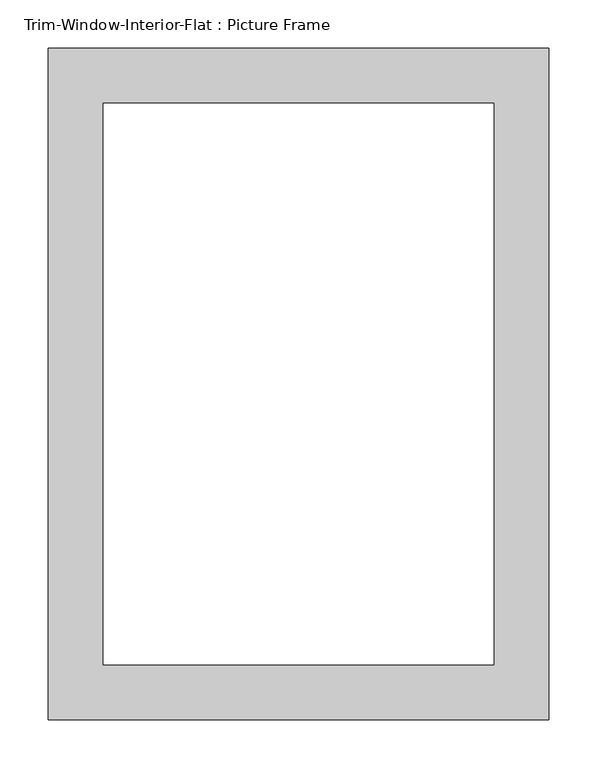
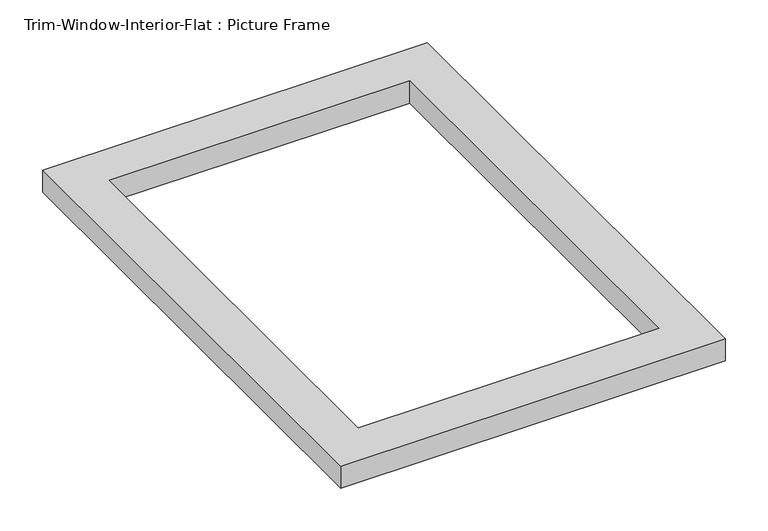
"""IFC4 building model written with IfcOpenShell, lengths in millimetres: proxy geometry, Trim-Window-Interior-Flat : Picture Frame."""

from ifc_helpers import new_model, si_unit, origin, origin_with_axes, place, context, project, spatial, polyline, outline, extrude, source, transform, mapped, element, save


def trim_window_interior_flat_picture_frame_58837336(model_context):
    return source(origin(), model_context, "Body", "SweptSolid", [
        extrude(outline(polyline([(260.35, 44.45), (260.35, -654.05), (-260.35, -654.05), (-260.35, 44.45), (260.35, 44.45)]), holes=[polyline([(203.2, -12.7), (-203.2, -12.7), (-203.2, -596.9), (203.2, -596.9), (203.2, -12.7)])]), origin_with_axes(), (0.0, 0.0, 1.0), 31.75),
    ])


if __name__ == "__main__":
    model = new_model("IFC4")
    model_context = context("Model", 3, world=origin())
    ifc_project = project(units=[si_unit("LENGTHUNIT", "METRE", prefix="MILLI")], contexts=[model_context])
    site = spatial("IfcSite", under=ifc_project)
    building = spatial("IfcBuilding", under=site)
    placement = place(None, origin())
    trim_window_interior_flat_picture_frame_shape = trim_window_interior_flat_picture_frame_58837336(model_context)
    element("IfcBuildingElementProxy", 1, Name="Trim-Window-Interior-Flat : Picture Frame", ObjectType="Trim-Window-Interior-Flat : Picture Frame", at=placement, inside=building, context=model_context, shape_type="MappedRepresentation", body=[
        mapped(trim_window_interior_flat_picture_frame_shape, transform((0.0, 0.0, 0.0), x_axis=(1.0, 0.0, 0.0), y_axis=(0.0, 1.0, 0.0), z_axis=(0.0, 0.0, 1.0))),
    ])
    save(model, "model.ifc")

# Revit data of these elements
# Type "Trim-Window-Interior-Flat : Picture Frame"
#   Trim Thickness_Picture Frame = 0' - 1 1/4"
#   Trim Width = 0' - 2 1/4"
#   Trim Thickness_with Sill = 0' - 0 3/4"
#   Sill Thickness = 0' - 1 1/4"
#   Opening Width [instance default] = 2' - 0"
#   Opening Height [instance default] = 3' - 0"
#   Default Elevation = 4' - 0"
#   Sill = no
#   Picture Frame = yes
#   Trim Material [instance default] = none
# Element 1 (IfcBuildingElementProxy, "Trim-Window-Interior-Flat : Picture Frame")
#   Opening Width = 1' - 5"
#   Opening Height = 2' - 0"
#   Trim Material = Wood - Stained
#   Materials on its faces: "Wood - Stained"
# Materials
#   "Wood - Stained": class "Wood", colour RGB 224 178 126, transparency 0, Cost = 0
